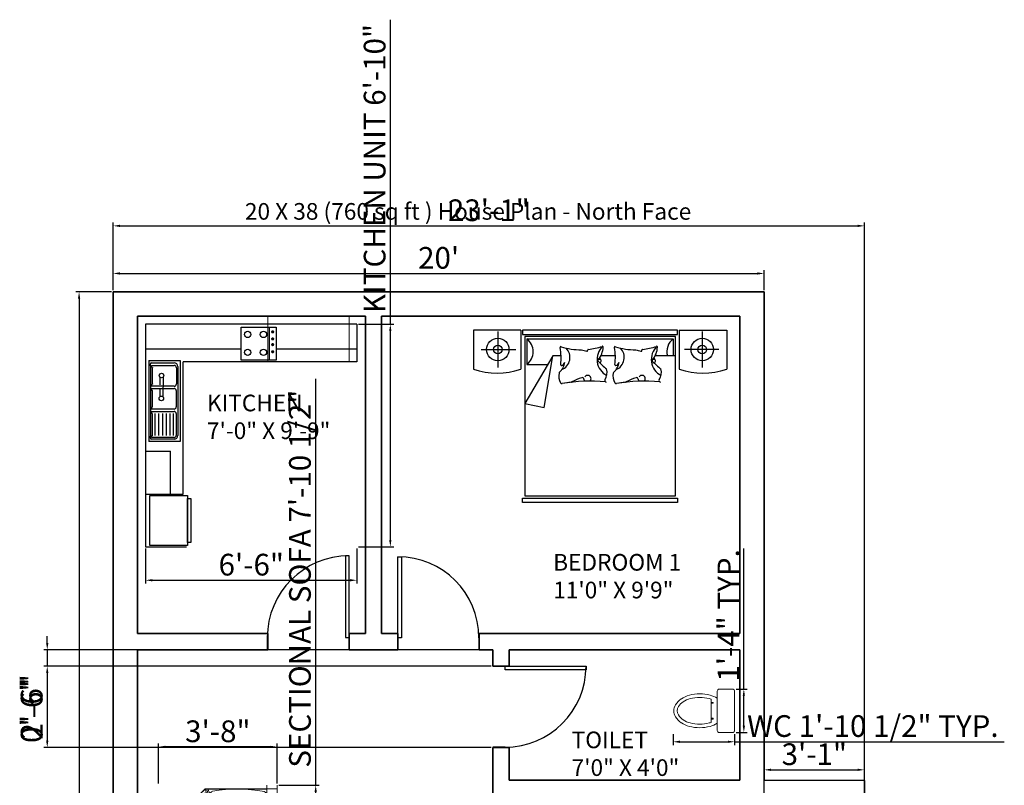
# Model space of a CAD drawing. Units: inches. Extents: x 3064 to 3427, y 2432 to 3115.
# Tile 3 of 3: x 3064 to 3427, y 2833 to 3115. Entities that reach past the tile are written whole.
import ezdxf

# ---------------------------------------------------------------- set-up
doc = ezdxf.new("R2010")
doc.units = ezdxf.units.IN
for name, color, linetype, lineweight in [('A-ANNO-DIMS', 2, 'Continuous', 13), ('A-ANNO-TEXT', 7, 'Continuous', 25), ('A-AREA-IDEN', 7, 'Continuous', 18), ('A-DOOR', 4, 'Continuous', 25), ('A-WALL', 7, 'Continuous', 35), ('FUR', 42, 'Continuous', 18), ('THIET-BI', 21, 'Continuous', 18)]:
    doc.layers.add(name, color=color, linetype=linetype, lineweight=lineweight)
for name, color, linetype in [('HID', 11, 'Continuous'), ('SAN', 5, 'Continuous'), ('TEFRIŞ', 11, 'Continuous'), ('wood', 26, 'Continuous')]:
    doc.layers.add(name, color=color, linetype=linetype)
doc.styles.get("Standard").update_dxf_attribs({"font": 'arial.ttf'})
doc.dimstyles.new('ISO-25', dxfattribs={"dimtxt": 8, "dimasz": 2.5, "dimexe": 1.25, "dimexo": 0.625, "dimtad": 1, "dimdec": 0, "dimlunit": 4, "dimtxsty": 'Standard', "dimcen": 2.5, "dimadec": 0, "dimazin": 0, "dimtfac": 1, "dimtdec": 0, "dimtmove": 0, "dimatfit": 3, "dimfxl": 1, "dimarcsym": 0})

# ---------------------------------------------------------------- blocks, each defined once
blk = doc.blocks.new('A$C008029BD')
at = {"layer": 'TEFRIŞ', "ltscale": 0.05}
for p, q in [((0, 0), (0, -3.55)), ((3.37, 0), (0, 0)), ((3.37, 0), (3.37, -0.6)), ((1.522, -0.4), (0, -0.4)), ((3.37, -0.4), (2.083, -0.4)), ((0.05, -0.581), (0.05, -1.869)), ((0.05, -0.581), (0.55, -0.581)), ((0.096, -0.617), (0.454, -0.617)), ((0.55, -0.581), (0.55, -1.869)), ((0.6, -2.71), (0.6, -0.6)), ((3.37, -0.6), (0.6, -0.6)), ((0.086, -1.773), (0.086, -0.677)), ((0.099, -0.659), (0.457, -0.659)), ((0.113, -0.954), (0.113, -0.695)), ((0.493, -0.695), (0.493, -0.954)), ((0.514, -0.677), (0.514, -1.773)), ((0.23, -0.846), (0.229, -0.967)), ((0.28, -0.846), (0.277, -1.158)), ((0.096, -1.024), (0.454, -1.024)), ((0.457, -0.99), (0.099, -0.99)), ((0.11, -1.319), (0.11, -1.06)), ((0.228, -1.02), (0.227, -1.159)), ((0.49, -1.06), (0.49, -1.319)), ((0.454, -1.355), (0.096, -1.355)), ((0.096, -1.391), (0.454, -1.391)), ((0.11, -1.773), (0.11, -1.427)), ((0.154, -1.773), (0.154, -1.427)), ((0.214, -1.773), (0.214, -1.427)), ((0.274, -1.773), (0.274, -1.427)), ((0.334, -1.773), (0.334, -1.427)), ((0.39, -1.773), (0.39, -1.427)), ((0.444, -1.773), (0.444, -1.427)), ((0.49, -1.427), (0.49, -1.773)), ((0.55, -1.869), (0.05, -1.869)), ((0.454, -1.809), (0.096, -1.809)), ((0.454, -1.833), (0.096, -1.833)), ((0, -2.025), (0.4, -2.025)), ((0.4, -2.71), (0.4, -2.025)), ((0, -2.71), (0.6, -2.71)), ((0, -3.55), (0.65, -3.55))]:
    blk.add_line(p, q, dxfattribs=at)
at = {"layer": 'TEFRIŞ'}
blk.add_line((1.969, -0.05), (1.969, -0.572), dxfattribs=at)
at = {"layer": 'TEFRIŞ', "ltscale": 0.05}
for points in [[(1.522, -0.05), (2.083, -0.05), (2.083, -0.572), (1.522, -0.572)], [(0.67, -2.73), (0.67, -3.53), (0.07, -3.53), (0.07, -2.73)], [(0.72, -2.78), (0.72, -3.48), (0.67, -3.48), (0.67, -2.78)]]:
    blk.add_lwpolyline(points, close=True, dxfattribs=at)
at = {"layer": 'TEFRIŞ', "const_width": 0.025}
for points in [[(2.014, -0.123, 1), (2.039, -0.123, 1)], [(2.014, -0.236, 1), (2.039, -0.236, 1)], [(2.014, -0.327, 1), (2.039, -0.327, 1)], [(2.014, -0.44, 1), (2.039, -0.44, 1)]]:
    blk.add_lwpolyline(points, format="xyb", close=True, dxfattribs=at)
at = {"layer": 'TEFRIŞ', "ltscale": 0.05}
for centre, radius in [((1.628, -0.164), 0.0505), ((1.628, -0.45), 0.0505), ((0.255, -0.82), 0.036), ((0.252, -1.184), 0.036)]:
    blk.add_circle(centre, radius, dxfattribs=at)
at = {"layer": 'TEFRIŞ'}
for centre in [(1.88, -0.164), (1.88, -0.45)]:
    blk.add_circle(centre, 0.0505, dxfattribs=at)
at = {"layer": 'TEFRIŞ', "ltscale": 0.05}
for centre, radius, start, end in [((0.108, -0.649), 0.0351, 110.4976, 230.5777), ((0.454, -0.677), 0.06, 0, 90), ((0.118, -0.673), 0.023, 143.9853, 258.5157), ((0.457, -0.695), 0.036, 0, 90), ((0.115, -1.038), 0.023, 143.9853, 258.5157), ((0.118, -0.976), 0.023, 101.4843, 216.0147), ((0.454, -1.06), 0.036, 0, 90), ((0.457, -0.954), 0.036, 270, 0), ((0.115, -1.341), 0.023, 101.4843, 216.0147), ((0.115, -1.405), 0.023, 143.9853, 258.5157), ((0.454, -1.319), 0.036, 270, 0), ((0.454, -1.427), 0.036, 0, 90), ((0.108, -1.801), 0.0351, 129.4223, 249.5024), ((0.115, -1.796), 0.023, 101.4843, 216.0147), ((0.454, -1.773), 0.06, 270, 0), ((0.454, -1.773), 0.036, 270, 0)]:
    blk.add_arc(centre, radius, start, end, dxfattribs=at)
blk = doc.blocks.new('A$C47AC156F')
at = {"layer": 'HID'}
for centre, radius, start, end in [((1.015, 1.799), 0.00933, 72.7248, 190.959), ((0.396, 1.679), 0.622, 352.7363, 10.959), ((1.25, 2.553), 0.781, 252.7248, 270.2702), ((0.966, 1.684), 0.155, 292.7628, 43.8922), ((1.385, 2.121), 0.373, 249.4168, 259.3085), ((1.317, 1.764), 0.00933, 259.3085, 10.689), ((1.336, 1.768), 0.00933, 96.2196, 190.689), ((1.25, 2.553), 0.781, 276.2196, 288.2114), ((1.645, 1.66), 0.21, 133.8947, 242.3952), ((1.258, 1.815), 0.249, 319.9211, 357.124), ((1.497, 1.803), 0.00933, 357.124, 108.2114), ((1.497, 1.803), 0.00933, 357.124, 108.2114), ((1.645, 1.799), 0.00933, 72.7248, 190.959), ((1.026, 1.679), 0.622, 352.7363, 10.959), ((1.88, 2.553), 0.781, 252.7248, 270.2702), ((1.596, 1.684), 0.155, 292.7628, 43.8922), ((2.015, 2.121), 0.373, 249.4168, 259.3085), ((1.947, 1.764), 0.00933, 259.3085, 10.689), ((1.966, 1.768), 0.00933, 96.2196, 190.689), ((1.88, 2.553), 0.781, 276.2196, 288.2114), ((2.275, 1.66), 0.21, 133.8947, 242.3952), ((1.888, 1.815), 0.249, 319.9211, 357.124), ((2.127, 1.803), 0.00933, 357.124, 108.2114), ((2.127, 1.803), 0.00933, 357.124, 108.2114), ((0.871, 1.658), 0.194, 311.6071, 349.7845), ((1.005, 1.648), 0.0615, 288.2985, 335.7891), ((1.453, 1.646), 0.00933, 118.8315, 225.8329), ((2.727, 2.958), 1.838, 225.8329, 230.0245), ((0.994, -0.376), 2.088, 76.4982, 77.2888), ((0.994, 3.644), 2.088, 282.7018, 282.7206), ((1.445, 1.644), 0.0373, 312.662, 59.1573), ((1.501, 1.658), 0.194, 311.6071, 349.7845), ((1.635, 1.648), 0.0615, 288.2985, 335.7891), ((2.083, 1.646), 0.00933, 118.8315, 225.8329), ((3.357, 2.958), 1.838, 225.8329, 230.0245), ((1.624, -0.376), 2.088, 76.4982, 77.2888), ((1.624, 3.644), 2.088, 282.7018, 282.7206), ((2.075, 1.644), 0.0373, 312.662, 59.1573), ((1.142, 1.469), 0.152, 167.3377, 211.666), ((1.012, 1.499), 0.0187, 131.6071, 167.3377), ((1.022, 1.599), 0.00933, 172.7363, 288.2985), ((1.401, 1.508), 0.151, 327.1663, 15.7613), ((1.772, 1.469), 0.152, 167.3377, 211.666), ((1.642, 1.499), 0.0187, 131.6071, 167.3377), ((1.652, 1.599), 0.00933, 172.7363, 288.2985), ((2.031, 1.508), 0.151, 327.1663, 15.7613), ((1.028, 1.399), 0.0187, 211.666, 279.4465), ((1.35, -0.534), 1.941, 84.5852, 99.4465), ((1.35, -0.534), 1.941, 96.386, 99.4465), ((1.132, 1.414), 0.0187, 276.386, 303.7955), ((1.54, 0.631), 0.864, 109.049, 117.3823), ((1.264, 1.43), 0.0187, 2.6426, 109.049), ((1.301, 1.432), 0.0187, 182.6426, 192.7015), ((1.323, 1.437), 0.0414, 192.7015, 227.1556), ((1.326, 1.436), 0.0395, 312.3565, 145.7762), ((1.543, 1.416), 0.0187, 147.1663, 264.3422), ((1.659, 1.399), 0.0187, 211.666, 279.4465), ((1.98, -0.534), 1.941, 84.5852, 99.4465), ((1.98, -0.534), 1.941, 96.386, 99.4465), ((1.762, 1.414), 0.0187, 276.386, 303.7955), ((2.17, 0.631), 0.864, 109.049, 117.3823), ((1.894, 1.43), 0.0187, 2.6426, 109.049), ((1.931, 1.432), 0.0187, 182.6426, 192.7015), ((1.954, 1.437), 0.0414, 192.7015, 227.1556), ((1.956, 1.436), 0.0395, 312.3565, 145.7762), ((2.173, 1.416), 0.0187, 147.1663, 264.3422)]:
    blk.add_arc(centre, radius, start, end, dxfattribs=at)
at = {"layer": 'SAN'}
for p, q in [((0.283, 1.985), (0.283, 1.566)), ((2.657, 1.985), (2.657, 1.566)), ((0.09, 1.775), (0.491, 1.775)), ((2.85, 1.775), (2.449, 1.775))]:
    blk.add_line(p, q, dxfattribs=at)
for centre, radius in [((0.283, 1.775), 0.13), ((2.657, 1.775), 0.13), ((0.283, 1.775), 0.05), ((2.657, 1.775), 0.05)]:
    blk.add_circle(centre, radius, dxfattribs=at)
at = {"layer": 'wood'}
for p, q in [((0, 1.998), (0, 1.548)), ((0.55, 1.998), (0, 1.998)), ((0.55, 1.998), (0.55, 1.548)), ((2.39, 1.998), (2.94, 1.998)), ((2.39, 1.998), (2.39, 1.548)), ((2.94, 1.998), (2.94, 1.548)), ((0.62, 1.9), (2.32, 1.9)), ((0.62, 1.9), (0.62, 1.6)), ((2.32, 1.9), (2.32, 1.7)), ((0.92, 1.7), (0.595, 1.15)), ((0.82, 1.1), (0.92, 1.7)), ((1.017, 1.7), (0.92, 1.7)), ((1.647, 1.7), (1.479, 1.7)), ((2.345, 1.7), (2.109, 1.7)), ((0.62, 1.6), (0.861, 1.6)), ((0.595, 1.15), (0.82, 1.1))]:
    blk.add_line(p, q, dxfattribs=at)
for points in [[(0.57, 1.95), (2.37, 1.95), (2.37, 2), (0.57, 2)], [(2.345, 0.075), (2.345, 1.925), (0.595, 1.925), (0.595, 0.075)], [(0.57, 0.05), (2.37, 0.05), (2.37, 0), (0.57, 0)]]:
    blk.add_lwpolyline(points, close=True, dxfattribs=at)
for centre, radius, start, end in [((0.504, 1.75), 0.19, 307.7826, 52.2174), ((2.436, 1.75), 0.19, 127.7826, 195.2747), ((0.275, 2.342), 0.84, 250.89, 289.11), ((2.665, 2.342), 0.84, 250.89, 289.11)]:
    blk.add_arc(centre, radius, start, end, dxfattribs=at)
blk = doc.blocks.new('A$C5B9B1B1E')
at = {"layer": 'FUR'}
for p, q in [((0.68, 1.857), (3.32, 1.857)), ((0.044, 1.127), (0.687, 1.804)), ((0.046, 1.126), (0.691, 1.805)), ((0.687, 1.804), (3.246, 1.804)), ((0.689, 1.807), (3.298, 1.807)), ((0.718, 1.807), (1.035, 0.991)), ((0.741, 1.807), (0.774, 1.719)), ((1.587, 1.804), (1.587, 1.757)), ((1.608, 1.804), (1.608, 1.041)), ((1.629, 1.804), (1.629, 1.757)), ((2.343, 1.804), (2.343, 1.041)), ((2.364, 1.804), (2.364, 1.041)), ((2.385, 1.804), (2.385, 1.757)), ((3.27, 1.807), (2.952, 0.991)), ((3.247, 1.807), (3.213, 1.719)), ((3.942, 1.126), (3.296, 1.805)), ((3.944, 1.127), (3.298, 1.807)), ((0.748, 1.672), (1.007, 1.005)), ((0.792, 1.675), (1.057, 0.993)), ((1.587, 1.671), (1.587, 1.041)), ((1.603, 1.671), (1.603, 1.041)), ((1.629, 1.671), (1.629, 1.041)), ((2.385, 1.671), (2.385, 1.041)), ((3.196, 1.675), (2.93, 0.993)), ((3.24, 1.672), (2.98, 1.005)), ((0.044, 1.127), (0.044, 0)), ((0.044, 1.127), (0.112, 1.103)), ((0.044, 1.105), (0.856, 0.808)), ((0.044, 1.083), (0.133, 1.05)), ((0.046, 1.082), (0.046, 0.164)), ((0.181, 1.077), (0.842, 0.836)), ((3.944, 1.105), (3.131, 0.808)), ((3.807, 1.077), (3.145, 0.836)), ((3.944, 1.083), (3.854, 1.05)), ((3.944, 1.127), (3.875, 1.103)), ((3.941, 1.082), (3.941, 0.164)), ((3.944, 1.127), (3.944, 0)), ((0.167, 1.038), (0.86, 0.785)), ((0.997, 0.952), (0.895, 0.848)), ((2.991, 0.952), (3.093, 0.848)), ((3.82, 1.038), (3.128, 0.785)), ((0, 0.164), (0.663, 0.164)), ((4, 0.164), (3.325, 0.164)), ((0, 0), (0.775, 0)), ((4, 0), (3.219, 0))]:
    blk.add_line(p, q, dxfattribs=at)
for centre, radius, start, end in [((1.999, -0.1), 2.263, 125.9311, 146.4201), ((0.827, 1.714), 0.0525, 104.0803, 255.9197), ((1.2, -0.267), 2.068, 79.3218, 100.7558), ((1.571, 1.714), 0.0529, 283.4421, 76.5579), ((1.661, 1.714), 0.0529, 103.4421, 256.5579), ((1.974, 0.302), 1.499, 77.3591, 102.5496), ((2.289, 1.714), 0.0525, 284.0803, 75.9197), ((2.417, 1.714), 0.0529, 103.4421, 256.5579), ((2.788, -0.267), 2.068, 79.2442, 100.6782), ((3.161, 1.714), 0.0525, 284.0803, 75.9197), ((1.989, -0.1), 2.263, 33.5799, 54.0689), ((-2.245, 3.806), 3.68, 319.5649, 324.3474), ((-2.245, 3.806), 3.733, 320.6889, 324.3474), ((1.373, 5.964), 4.337, 262.5873, 266.2564), ((1.493, 7.461), 5.886, 263.3874, 265.2569), ((1.257, 3.126), 1.499, 272.4014, 282.5496), ((1.257, 3.126), 1.551, 272.4014, 282.5496), ((1.974, 3.126), 1.551, 257.1404, 261.9048), ((1.974, 3.126), 1.499, 257.4504, 262.6454), ((1.974, 3.126), 1.499, 274.5548, 275.3997), ((1.974, 3.126), 1.499, 278.9885, 282.6409), ((1.974, 3.126), 1.551, 280.7847, 283.7486), ((2.73, 3.126), 1.551, 257.4504, 267.5986), ((2.73, 3.126), 1.499, 257.4504, 267.5986), ((2.614, 5.964), 4.337, 273.7436, 277.4127), ((2.494, 7.461), 5.886, 274.7431, 276.6126), ((6.233, 3.806), 3.733, 215.6526, 219.3111), ((6.233, 3.806), 3.68, 215.6526, 220.4351), ((0.159, 1.125), 0.0525, 149.9951, 301.8345), ((-0.635, 2.334), 1.499, 303.2739, 311.5982), ((-0.635, 2.334), 1.551, 304.4606, 312.1941), ((4.623, 2.334), 1.551, 227.8059, 235.5394), ((4.623, 2.334), 1.499, 228.4018, 236.7261), ((3.828, 1.125), 0.0525, 238.1655, 30.0049), ((2.31, 0.617), 2.263, 170.0163, 190.5053), ((0.133, 0.997), 0.0529, 13.4421, 166.5579), ((-3.456, 0.47), 3.68, 1.9572, 8.4326), ((-3.456, 0.47), 3.733, 1.9572, 8.4326), ((0.961, 0.987), 0.05, 315.6002, 21.264), ((1.299, 2.034), 1.068, 256.9274, 284.5801), ((1.545, 1.041), 0.042, 279.7794, 0), ((1.561, 1.041), 0.042, 279.7794, 0), ((1.671, 1.041), 0.042, 180, 260.2206), ((1.986, 2.869), 1.897, 260.2206, 279.7794), ((2.301, 1.041), 0.042, 279.7794, 0), ((2.427, 1.041), 0.042, 180, 260.2206), ((2.689, 2.034), 1.068, 255.4199, 283.0726), ((3.027, 0.987), 0.05, 158.736, 224.3998), ((7.443, 0.47), 3.733, 171.5674, 178.0428), ((7.443, 0.47), 3.68, 171.5674, 178.0428), ((3.854, 0.997), 0.0529, 13.4421, 166.5579), ((1.678, 0.617), 2.263, 349.4947, 9.9837), ((-1.061, 0.519), 1.939, 345.4239, 7.8665), ((0.859, 0.883), 0.05, 249.9365, 315.6002), ((3.128, 0.883), 0.05, 224.3998, 290.0635), ((5.006, 0.521), 1.897, 172.0077, 194.7607), ((-1.275, 0.533), 1.499, 347.3591, 353.601), ((5.263, 0.533), 1.499, 186.399, 192.6409), ((0.136, 0.218), 0.0525, 194.0803, 345.9197), ((-1.275, 0.533), 1.551, 346.2514, 350.7022), ((0.643, 0.074), 0.0918, 328.6411, 77.5888), ((3.345, 0.074), 0.0918, 102.4112, 211.3589), ((5.263, 0.533), 1.551, 189.2978, 193.7486), ((3.851, 0.218), 0.0525, 194.0803, 345.9197), ((0.665, 0.069), 0.0703, 279.5212, 322.6757), ((0.775, 0.042), 0.042, 270, 345.2393), ((3.226, 0.057), 0.0573, 199.356, 262.7582), ((3.338, 0.086), 0.0936, 219.4969, 247.1448)]:
    blk.add_arc(centre, radius, start, end, dxfattribs=at)
at = {"layer": 'HID'}
for centre, radius, start, end in [((1.056, 2.162), 0.527, 287.478, 299.4698), ((1.393, 1.632), 0.104, 135.6927, 273.5175), ((1.159, 1.674), 0.168, 330.4242, 8.3824), ((1.319, 1.698), 0.0063, 8.3824, 119.4698), ((1.664, 1.652), 0.142, 287.6048, 36.1053), ((1.94, 1.709), 0.168, 172.876, 210.0789), ((1.78, 1.729), 0.0063, 61.7886, 172.876), ((1.78, 1.729), 0.0063, 61.7886, 172.876), ((2.032, 2.199), 0.527, 241.7886, 253.7804), ((1.883, 1.687), 0.0063, 339.311, 73.7804), ((2.283, 1.626), 0.168, 151.6176, 189.5758), ((2.141, 1.703), 0.0063, 40.5302, 151.6176), ((2.546, 2.05), 0.527, 220.5302, 232.522), ((2.594, 1.632), 0.104, 266.4825, 44.3073), ((2.829, 1.674), 0.168, 171.6176, 209.5758), ((2.669, 1.698), 0.0063, 60.5302, 171.6176), ((2.931, 2.162), 0.527, 240.5302, 252.522), ((1, 1.632), 0.0063, 83.9832, 202.2174), ((0.606, 1.471), 0.42, 3.9947, 22.2174), ((1.056, 2.162), 0.527, 263.9832, 281.5286), ((0.982, 1.549), 0.105, 304.0212, 55.1506), ((1.202, 1.894), 0.252, 260.6752, 270.5669), ((1.205, 1.649), 0.0063, 270.5669, 21.9475), ((1.216, 1.653), 0.0063, 107.478, 201.9475), ((1.31, 1.588), 0.0063, 150.4242, 237.1103), ((1.981, 2.625), 1.241, 237.1103, 241.1368), ((1.379, 1.514), 0.0244, 343.8009, 85.0524), ((1.809, 1.522), 0.102, 154.2387, 202.8337), ((1.795, 1.618), 0.0252, 110.8427, 217.338), ((1.859, 0.222), 1.409, 92.7112, 93.5018), ((2.33, 2.894), 1.409, 247.2794, 247.2982), ((1.791, 1.62), 0.0063, 304.1671, 51.1685), ((1.895, 1.683), 0.0063, 159.311, 270.6915), ((1.892, 1.928), 0.252, 270.6915, 280.5832), ((2.032, 2.199), 0.527, 259.7298, 277.2752), ((2.009, 1.552), 0.0126, 176.1991, 230.6607), ((2.302, 1.91), 0.476, 230.6607, 243.8744), ((2.119, 1.588), 0.105, 126.1078, 237.2372), ((2.088, 1.569), 0.0416, 194.2109, 241.7015), ((2.179, 1.559), 0.131, 180.2155, 218.3929), ((2.072, 1.538), 0.0063, 241.7015, 357.2637), ((2.497, 1.518), 0.42, 159.041, 177.2637), ((2.099, 1.67), 0.0063, 339.041, 97.2752), ((2.111, 1.597), 0.0063, 282.8897, 9.5758), ((2.231, 1.618), 0.0063, 138.0525, 249.4331), ((2.222, 1.627), 0.0063, 318.0525, 52.522), ((2.317, 1.848), 0.252, 249.4331, 259.3248), ((2.546, 2.05), 0.527, 238.4714, 256.0168), ((2.406, 1.449), 0.105, 104.8494, 215.9788), ((2.417, 1.532), 0.0063, 317.7826, 76.0168), ((2.608, 1.514), 0.0244, 94.9476, 196.1991), ((2.007, 2.625), 1.241, 298.8632, 302.8897), ((2.677, 1.588), 0.0063, 302.8897, 29.5758), ((2.771, 1.653), 0.0063, 338.0525, 72.522), ((2.783, 1.649), 0.0063, 158.0525, 269.4331), ((2.785, 1.894), 0.252, 269.4331, 279.3248), ((2.931, 2.162), 0.527, 258.4714, 276.0168), ((3.005, 1.549), 0.105, 124.8494, 235.9788), ((3.382, 1.471), 0.42, 157.7826, 176.0053), ((2.987, 1.632), 0.0063, 337.7826, 96.0168), ((0.277, 1.564), 0.252, 306.59, 316.4817), ((0.459, 1.407), 0.0063, 153.3928, 247.8623), ((-0.018, 1.646), 0.527, 333.3928, 345.3846), ((0.455, 1.395), 0.0063, 316.4817, 67.8623), ((0.498, 1.511), 0.0063, 54.2972, 165.3846), ((0.598, 1.519), 0.104, 181.6075, 319.4323), ((0.404, 1.38), 0.168, 16.339, 54.2972), ((0.571, 1.429), 0.0063, 196.339, 283.0251), ((0.293, 2.632), 1.241, 283.0251, 287.0516), ((0.263, 1.627), 0.476, 322.0404, 335.2541), ((0.673, 1.427), 0.0244, 29.7157, 130.9672), ((0.683, 1.433), 0.0126, 335.2541, 29.7157), ((1.031, 1.5), 0.0063, 183.9947, 299.557), ((1.013, 1.531), 0.0416, 299.557, 347.0475), ((0.923, 1.519), 0.131, 329.5087, 1.0429), ((1.135, 1.458), 0.099, 182.7962, 207.1304), ((1.058, 1.418), 0.0126, 207.1304, 290.9482), ((1.531, 0.183), 1.31, 105.1521, 110.9482), ((1.185, 1.46), 0.0126, 285.1521, 322.4345), ((1.324, 1.352), 0.163, 100.921, 142.4345), ((1.274, 1.728), 0.252, 258.5381, 270.9308), ((1.286, 1.487), 0.0126, 131.4659, 280.4525), ((1.185, 1.602), 0.141, 311.4659, 320.8131), ((1.237, 1.948), 0.476, 276.1256, 289.3393), ((1.391, 1.511), 0.0126, 289.3393, 343.8009), ((1.704, 1.478), 0.0126, 265.6578, 22.8337), ((1.603, 0.159), 1.31, 70.5535, 85.4148), ((1.85, 1.466), 0.0267, 24.2238, 217.6435), ((1.852, 1.466), 0.0279, 302.8444, 337.2985), ((1.866, 1.46), 0.0126, 337.2985, 347.3574), ((1.891, 1.454), 0.0126, 60.951, 167.3574), ((1.614, 0.955), 0.583, 52.6177, 60.951), ((1.977, 1.428), 0.0126, 226.2045, 253.614), ((1.603, 0.159), 1.31, 70.5535, 73.614), ((2.044, 1.406), 0.0126, 250.5535, 318.334), ((1.976, 1.466), 0.103, 318.334, 2.6623), ((2.067, 1.47), 0.0126, 2.6623, 38.3929), ((2.099, 1.494), 0.0126, 239.5475, 28.5341), ((2.234, 1.567), 0.141, 199.1869, 208.5341), ((2.017, 1.381), 0.163, 17.5655, 59.079), ((2.193, 1.717), 0.252, 249.0692, 261.4619), ((2.185, 1.434), 0.0126, 197.5655, 234.8479), ((1.423, 0.352), 1.31, 49.0518, 54.8479), ((2.452, 1.4), 0.131, 158.9571, 190.4913), ((2.371, 1.442), 0.0416, 172.9525, 220.443), ((2.344, 1.419), 0.0063, 220.443, 336.0053), ((2.733, 1.246), 0.42, 137.7826, 156.0053), ((2.597, 1.511), 0.0126, 196.1991, 250.6607), ((2.75, 1.948), 0.476, 250.6607, 263.8744), ((2.663, 1.352), 0.163, 37.5655, 79.079), ((2.803, 1.602), 0.141, 219.1869, 228.5341), ((2.702, 1.487), 0.0126, 259.5475, 48.5341), ((2.713, 1.728), 0.252, 269.0692, 281.4619), ((2.803, 1.46), 0.0126, 217.5655, 254.8479), ((2.457, 0.183), 1.31, 69.0518, 74.8479), ((2.93, 1.418), 0.0126, 249.0518, 332.8696), ((3.065, 1.519), 0.131, 178.9571, 210.4913), ((2.974, 1.531), 0.0416, 192.9525, 240.443), ((2.853, 1.458), 0.099, 332.8696, 357.2038), ((2.957, 1.5), 0.0063, 240.443, 356.0053), ((3.304, 1.433), 0.0126, 150.2843, 204.7459), ((3.315, 1.427), 0.0244, 49.0328, 150.2843), ((3.725, 1.627), 0.476, 204.7459, 217.9596), ((3.389, 1.519), 0.104, 220.5677, 358.3925), ((3.694, 2.632), 1.241, 252.9484, 256.9749), ((3.416, 1.429), 0.0063, 256.9749, 343.661), ((3.583, 1.38), 0.168, 125.7028, 163.661), ((4.005, 1.646), 0.527, 194.6154, 206.6072), ((3.533, 1.395), 0.0063, 112.1377, 223.5183), ((3.711, 1.564), 0.252, 223.5183, 233.41), ((3.528, 1.407), 0.0063, 292.1377, 26.6072), ((0.371, 1.166), 0.105, 349.936, 101.0654), ((1.734, 0.609), 1.31, 151.0669, 156.863), ((0.751, 1.275), 0.163, 146.8358, 188.3493), ((0.446, 1.501), 0.252, 304.4529, 316.8456), ((0.577, 1.249), 0.0126, 331.0669, 8.3493), ((0.474, 1.348), 0.141, 357.3807, 6.7279), ((0.627, 1.341), 0.0126, 177.3807, 326.3673), ((2.29, 1.351), 0.0126, 229.0518, 312.8696), ((2.232, 1.415), 0.099, 312.8696, 337.2038), ((3.36, 1.341), 0.0126, 213.6327, 2.6193), ((3.542, 1.501), 0.252, 223.1544, 235.5471), ((3.513, 1.348), 0.141, 173.2721, 182.6193), ((3.237, 1.275), 0.163, 351.6507, 33.1642), ((3.411, 1.249), 0.0126, 171.6507, 208.9331), ((2.253, 0.609), 1.31, 23.137, 28.9331), ((3.616, 1.166), 0.105, 78.9346, 190.064), ((3.822, 0.841), 0.42, 111.8678, 130.0905), ((4.005, 1.646), 0.527, 212.5566, 230.102), ((0.44, 1.167), 0.0063, 229.9095, 345.4718), ((0.406, 1.176), 0.0416, 345.4718, 32.9623), ((0.351, 1.103), 0.131, 15.4235, 46.9577), ((0.543, 1.212), 0.099, 228.711, 253.0452), ((0.518, 1.129), 0.0126, 253.0452, 336.863), ((3.47, 1.129), 0.0126, 203.137, 286.9548), ((3.445, 1.212), 0.099, 286.9548, 311.289), ((3.636, 1.103), 0.131, 133.0423, 164.5765), ((3.582, 1.176), 0.0416, 147.0377, 194.5282), ((3.547, 1.167), 0.0063, 194.5282, 310.0905), ((0.219, 0.669), 0.104, 225.6927, 3.5175), ((-0.775, 1.256), 1.241, 327.1103, 331.1368), ((0.336, 0.655), 0.0244, 73.8009, 175.0524), ((0.34, 0.666), 0.0126, 19.3393, 73.8009), ((-0.097, 0.513), 0.476, 6.1256, 19.3393), ((4.085, 0.513), 0.476, 160.6607, 173.8744), ((3.648, 0.666), 0.0126, 106.1991, 160.6607), ((3.651, 0.655), 0.0244, 4.9476, 106.1991), ((3.769, 0.669), 0.104, 176.4825, 314.3073), ((4.762, 1.256), 1.241, 208.8632, 212.8897), ((0.152, 0.594), 0.0063, 98.3824, 209.4698), ((-0.312, 0.331), 0.527, 17.478, 29.4698), ((0.176, 0.434), 0.168, 60.4242, 98.3824), ((0.197, 0.492), 0.0063, 197.478, 291.9475), ((0.202, 0.48), 0.0063, 0.5669, 111.9475), ((-0.044, 0.478), 0.252, 350.6752, 0.5669), ((0.262, 0.586), 0.0063, 240.4242, 327.1103), ((0.498, 0.6), 0.163, 190.921, 232.4345), ((0.249, 0.46), 0.141, 41.4659, 50.8131), ((0.363, 0.561), 0.0126, 221.4659, 10.4525), ((0.122, 0.55), 0.252, 348.5381, 0.9308), ((0.391, 0.46), 0.0126, 15.1521, 52.4345), ((1.668, 0.806), 1.31, 195.1521, 200.9482), ((2.32, 0.806), 1.31, 339.0518, 344.8479), ((3.597, 0.46), 0.0126, 127.5655, 164.8479), ((3.49, 0.6), 0.163, 307.5655, 349.079), ((3.624, 0.561), 0.0126, 169.5475, 318.5341), ((3.866, 0.55), 0.252, 179.0692, 191.4619), ((3.739, 0.46), 0.141, 129.1869, 138.5341), ((3.726, 0.586), 0.0063, 212.8897, 299.5758), ((3.811, 0.434), 0.168, 81.6176, 119.5758), ((3.786, 0.48), 0.0063, 68.0525, 179.4331), ((4.031, 0.478), 0.252, 179.4331, 189.3248), ((3.791, 0.492), 0.0063, 248.0525, 342.522), ((4.3, 0.331), 0.527, 150.5302, 162.522), ((-0.312, 0.331), 0.527, 353.9832, 11.5286), ((0.301, 0.258), 0.105, 34.0212, 145.1506), ((0.319, 0.289), 0.0416, 29.557, 77.0475), ((0.331, 0.198), 0.131, 59.5087, 91.0429), ((0.35, 0.306), 0.0063, 273.9947, 29.557), ((0.393, 0.41), 0.099, 272.7962, 297.1304), ((0.432, 0.333), 0.0126, 297.1304, 20.9482), ((3.556, 0.333), 0.0126, 159.0518, 242.8696), ((3.595, 0.41), 0.099, 242.8696, 267.2038), ((3.657, 0.198), 0.131, 88.9571, 120.4913), ((3.687, 0.258), 0.105, 34.8494, 145.9788), ((3.638, 0.306), 0.0063, 150.443, 266.0053), ((3.668, 0.289), 0.0416, 102.9525, 150.443), ((4.3, 0.331), 0.527, 168.4714, 186.0168), ((0.219, 0.276), 0.0063, 173.9832, 292.2174), ((0.38, -0.119), 0.42, 93.9947, 112.2174), ((3.608, -0.119), 0.42, 67.7826, 86.0053), ((3.769, 0.276), 0.0063, 247.7826, 6.0168)]:
    blk.add_arc(centre, radius, start, end, dxfattribs=at)
blk = doc.blocks.new('*D6')
at = {"layer": 'A-ANNO-DIMS', "color": 0, "lineweight": -2, "transparency": 16777216}
for p, q in [((3338.05, 2829.08), (3338.05, 2839.48)), ((3375.05, 2829.08), (3375.05, 2839.48)), ((3340.55, 2838.23), (3372.55, 2838.23))]:
    blk.add_line(p, q, dxfattribs=at)
at = {"layer": 'A-ANNO-DIMS', "color": 0, "transparency": 16777216}
for points in [[(3340.55, 2838.65), (3340.55, 2837.82), (3338.05, 2838.23)], [(3372.55, 2838.65), (3372.55, 2837.82), (3375.05, 2838.23)]]:
    blk.add_solid(points, dxfattribs=at)
at = {"layer": 'Defpoints', "color": 0, "transparency": 16777216}
for p in [(3375.05, 2838.23), (3338.05, 2828.45), (3375.05, 2828.45)]:
    blk.add_point(p, dxfattribs=at)
at = {"layer": 'A-ANNO-DIMS', "color": 0, "transparency": 16777216, "insert": (3356.55, 2842.95), "char_height": 8, "attachment_point": 5}
blk.add_mtext('3\'-1"', dxfattribs=at)
blk = doc.blocks.new('*U10')
for p, q in [((0, 0), (0, -6)), ((40, 0), (40, -6))]:
    blk.add_line(p, q)
blk.add_lwpolyline([(0, 0), (0, 40), (1.75, 40), (1.75, 0)], close=True)
blk.add_arc((0, 0), 40, 0, 90)
blk = doc.blocks.new('*U11')
for p, q in [((0, 0), (0, -6)), ((-40, 0), (-40, -6))]:
    blk.add_line(p, q)
blk.add_lwpolyline([(0, 0), (0, 40), (-1.75, 40), (-1.75, 0)], close=True)
blk.add_arc((0, 0), 40, 90, 180)
blk = doc.blocks.new('*U14')
for p, q in [((-40, 0), (-40, 6)), ((0, 0), (0, 6))]:
    blk.add_line(p, q)
blk.add_lwpolyline([(0, 0), (0, -40), (-1.75, -40), (-1.75, 0)], close=True)
blk.add_arc((0, 0), 40, 180, 270)
blk = doc.blocks.new('*D15')
at = {"layer": 'A-ANNO-DIMS', "color": 0, "lineweight": -2, "transparency": 16777216}
for p, q in [((3098.05, 3015.08), (3098.05, 3022.44)), ((3100.55, 3021.19), (3335.55, 3021.19)), ((3338.05, 3015.08), (3338.05, 3022.44))]:
    blk.add_line(p, q, dxfattribs=at)
at = {"layer": 'A-ANNO-DIMS', "color": 0, "transparency": 16777216}
for points in [[(3100.55, 3021.61), (3100.55, 3020.77), (3098.05, 3021.19)], [(3335.55, 3021.61), (3335.55, 3020.77), (3338.05, 3021.19)]]:
    blk.add_solid(points, dxfattribs=at)
at = {"layer": 'Defpoints', "color": 0, "transparency": 16777216}
for p in [(3338.05, 3021.19), (3098.05, 3014.45), (3338.05, 3014.45)]:
    blk.add_point(p, dxfattribs=at)
at = {"layer": 'A-ANNO-DIMS', "color": 0, "transparency": 16777216, "insert": (3218.05, 3025.9), "char_height": 8, "attachment_point": 5}
blk.add_mtext("20'", dxfattribs=at)
blk = doc.blocks.new('*D16')
at = {"layer": 'A-ANNO-DIMS', "color": 0, "lineweight": -2, "transparency": 16777216}
for p, q in [((3097.42, 3014.45), (3084.25, 3014.45)), ((3085.5, 3011.95), (3085.5, 2560.95)), ((3097.42, 2558.45), (3084.25, 2558.45))]:
    blk.add_line(p, q, dxfattribs=at)
at = {"layer": 'A-ANNO-DIMS', "color": 0, "transparency": 16777216}
for points in [[(3085.09, 3011.95), (3085.92, 3011.95), (3085.5, 3014.45)], [(3085.09, 2560.95), (3085.92, 2560.95), (3085.5, 2558.45)]]:
    blk.add_solid(points, dxfattribs=at)
at = {"layer": 'Defpoints', "color": 0, "transparency": 16777216}
for p in [(3098.05, 3014.45), (3085.5, 2558.45), (3098.05, 2558.45)]:
    blk.add_point(p, dxfattribs=at)
at = {"layer": 'A-ANNO-DIMS', "color": 0, "transparency": 16777216, "insert": (3080.79, 2786.45), "char_height": 8, "attachment_point": 5, "rotation": 90}
blk.add_mtext("38'", dxfattribs=at)
blk = doc.blocks.new('WC-TANK')
for p, q in [((16.04, 15.24), (16.04, 0.8)), ((21.66, 16.04), (16.85, 16.04)), ((22.46, 0.8), (22.46, 15.24)), ((13.79, 11.11), (13.79, 10.8)), ((14.52, 11.11), (13.79, 11.11)), ((13.8, 12.29), (13.8, 3.76)), ((14.52, 10.8), (14.52, 11.11)), ((13.79, 10.8), (14.52, 10.8)), ((13.79, 4.94), (13.79, 5.26)), ((13.79, 5.26), (14.52, 5.26)), ((14.52, 4.94), (13.79, 4.94)), ((14.52, 5.26), (14.52, 4.94)), ((16.85, 0), (21.66, 0))]:
    blk.add_line(p, q)
for centre, radius, start, end in [((16.85, 15.24), 0.802, 90, 180), ((21.66, 15.24), 0.802, 0, 90), ((6.75, 6.36), 7.24, 123.0315, 147.5002), ((6.75, 6.36), 5.95, 123.0315, 147.5002), ((8.47, 3.73), 10.38, 105.0731, 123.0315), ((8.47, 3.73), 9.1, 105.0731, 123.0315), ((9.59, -0.44), 14.7, 74.9269, 105.0732), ((9.59, -0.44), 13.41, 74.9269, 105.0732), ((10.71, 3.73), 9.1, 70.176, 74.9269), ((10.71, 3.73), 10.38, 59.0966, 74.9269), ((4.15, 8.02), 4.15, 147.5002, 212.4998), ((4.15, 8.02), 2.87, 147.5002, 212.4998), ((6.75, 9.68), 7.24, 212.4998, 236.9685), ((6.75, 9.68), 5.95, 212.4998, 236.9685), ((8.47, 12.31), 9.1, 236.9685, 254.9269), ((10.71, 12.31), 9.1, 285.0731, 289.824), ((8.47, 12.31), 10.38, 236.9685, 254.9269), ((9.59, 16.48), 14.7, 254.9269, 285.0731), ((9.59, 16.48), 13.41, 254.9269, 285.0731), ((10.71, 12.31), 10.38, 285.0731, 300.9034), ((16.85, 0.8), 0.802, 180, 270), ((21.66, 0.8), 0.802, 270, 0)]:
    blk.add_arc(centre, radius, start, end)
blk = doc.blocks.new('*D24')
at = {"layer": 'A-ANNO-DIMS', "color": 0, "lineweight": -2, "transparency": 16777216}
for p, q in [((3304.5, 2851.35), (3304.5, 2847.32)), ((3327.18, 2851.35), (3327.18, 2847.32)), ((3307, 2848.57), (3324.68, 2848.57)), ((3327.18, 2848.57), (3426.6, 2848.57))]:
    blk.add_line(p, q, dxfattribs=at)
at = {"layer": 'A-ANNO-DIMS', "color": 0, "transparency": 16777216}
for points in [[(3307, 2848.99), (3307, 2848.15), (3304.5, 2848.57)], [(3324.68, 2848.99), (3324.68, 2848.15), (3327.18, 2848.57)]]:
    blk.add_solid(points, dxfattribs=at)
at = {"layer": 'Defpoints', "color": 0, "transparency": 16777216}
for p in [(3304.5, 2851.97), (3327.18, 2851.97), (3327.18, 2848.57)]:
    blk.add_point(p, dxfattribs=at)
at = {"layer": 'A-ANNO-DIMS', "color": 0, "transparency": 16777216, "insert": (3378.14, 2853.33), "char_height": 8, "attachment_point": 5}
blk.add_mtext('WC 1\'-10 1/2" TYP.', dxfattribs=at)
blk = doc.blocks.new('*D25')
at = {"layer": 'A-ANNO-DIMS', "color": 0, "lineweight": -2, "transparency": 16777216}
for p, q in [((3330.58, 2868.02), (3330.58, 2919.78)), ((3327.8, 2868.02), (3331.83, 2868.02)), ((3330.58, 2854.47), (3330.58, 2865.52)), ((3327.8, 2851.97), (3331.83, 2851.97))]:
    blk.add_line(p, q, dxfattribs=at)
at = {"layer": 'A-ANNO-DIMS', "color": 0, "transparency": 16777216}
for points in [[(3330.16, 2865.52), (3330.99, 2865.52), (3330.58, 2868.02)], [(3330.16, 2854.47), (3330.99, 2854.47), (3330.58, 2851.97)]]:
    blk.add_solid(points, dxfattribs=at)
at = {"layer": 'Defpoints', "color": 0, "transparency": 16777216}
for p in [(3327.18, 2868.02), (3330.58, 2868.02), (3327.18, 2851.97)]:
    blk.add_point(p, dxfattribs=at)
at = {"layer": 'A-ANNO-DIMS', "color": 0, "transparency": 16777216, "insert": (3325.93, 2895.15), "char_height": 8, "attachment_point": 5, "rotation": 90}
blk.add_mtext('1\'-4" TYP.', dxfattribs=at)
blk = doc.blocks.new('*D26')
at = {"layer": 'A-ANNO-DIMS', "color": 0, "lineweight": -2, "transparency": 16777216}
for p, q in [((3200.25, 3002.51), (3200.25, 3114.72)), ((3188.56, 3002.51), (3201.5, 3002.51)), ((3200.25, 2922.92), (3200.25, 3000.01)), ((3188.56, 2920.42), (3201.5, 2920.42))]:
    blk.add_line(p, q, dxfattribs=at)
at = {"layer": 'A-ANNO-DIMS', "color": 0, "transparency": 16777216}
for points in [[(3199.83, 3000.01), (3200.66, 3000.01), (3200.25, 3002.51)], [(3199.83, 2922.92), (3200.66, 2922.92), (3200.25, 2920.42)]]:
    blk.add_solid(points, dxfattribs=at)
at = {"layer": 'Defpoints', "color": 0, "transparency": 16777216}
for p in [(3187.93, 3002.51), (3200.25, 3002.51), (3187.93, 2920.42)]:
    blk.add_point(p, dxfattribs=at)
at = {"layer": 'A-ANNO-DIMS', "color": 0, "transparency": 16777216, "insert": (3195.49, 3059.86), "char_height": 8, "attachment_point": 5, "rotation": 90}
blk.add_mtext('KITCHEN UNIT 6\'-10"', dxfattribs=at)
blk = doc.blocks.new('*D27')
at = {"layer": 'A-ANNO-DIMS', "color": 0, "lineweight": -2, "transparency": 16777216}
for p, q in [((3110.01, 2919.8), (3110.01, 2906.86)), ((3187.93, 2919.8), (3187.93, 2906.86)), ((3112.51, 2908.11), (3185.43, 2908.11))]:
    blk.add_line(p, q, dxfattribs=at)
at = {"layer": 'A-ANNO-DIMS', "color": 0, "transparency": 16777216}
for points in [[(3112.51, 2908.52), (3112.51, 2907.69), (3110.01, 2908.11)], [(3185.43, 2908.52), (3185.43, 2907.69), (3187.93, 2908.11)]]:
    blk.add_solid(points, dxfattribs=at)
at = {"layer": 'Defpoints', "color": 0, "transparency": 16777216}
for p in [(3110.01, 2920.42), (3187.93, 2920.42), (3187.93, 2908.11)]:
    blk.add_point(p, dxfattribs=at)
at = {"layer": 'A-ANNO-DIMS', "color": 0, "transparency": 16777216, "insert": (3148.97, 2912.82), "char_height": 8, "attachment_point": 5}
blk.add_mtext('6\'-6"', dxfattribs=at)
blk = doc.blocks.new('*D28')
at = {"layer": 'A-ANNO-DIMS', "color": 0, "lineweight": -2, "transparency": 16777216}
for p, q in [((3172.73, 2832.53), (3172.73, 2982.35)), ((3159.19, 2832.53), (3173.98, 2832.53)), ((3172.73, 2740.61), (3172.73, 2830.03)), ((3159.19, 2738.11), (3173.98, 2738.11))]:
    blk.add_line(p, q, dxfattribs=at)
at = {"layer": 'A-ANNO-DIMS', "color": 0, "transparency": 16777216}
for points in [[(3172.31, 2830.03), (3173.15, 2830.03), (3172.73, 2832.53)], [(3172.31, 2740.61), (3173.15, 2740.61), (3172.73, 2738.11)]]:
    blk.add_solid(points, dxfattribs=at)
at = {"layer": 'Defpoints', "color": 0, "transparency": 16777216}
for p in [(3158.57, 2832.53), (3172.73, 2832.53), (3158.57, 2738.11)]:
    blk.add_point(p, dxfattribs=at)
at = {"layer": 'A-ANNO-DIMS', "color": 0, "transparency": 16777216, "insert": (3167.96, 2908.69), "char_height": 8, "attachment_point": 5, "rotation": 90}
blk.add_mtext('SECTIONAL SOFA 7\'-10 1/2"', dxfattribs=at)
blk = doc.blocks.new('*D29')
at = {"layer": 'A-ANNO-DIMS', "color": 0, "lineweight": -2, "transparency": 16777216}
for p, q in [((3114.74, 2833.15), (3114.74, 2847.94)), ((3156.07, 2846.69), (3117.24, 2846.69)), ((3158.57, 2833.15), (3158.57, 2847.94))]:
    blk.add_line(p, q, dxfattribs=at)
at = {"layer": 'A-ANNO-DIMS', "color": 0, "transparency": 16777216}
for points in [[(3117.24, 2847.11), (3117.24, 2846.28), (3114.74, 2846.69)], [(3156.07, 2847.11), (3156.07, 2846.28), (3158.57, 2846.69)]]:
    blk.add_solid(points, dxfattribs=at)
at = {"layer": 'Defpoints', "color": 0, "transparency": 16777216}
for p in [(3114.74, 2846.69), (3114.74, 2832.53), (3158.57, 2832.53)]:
    blk.add_point(p, dxfattribs=at)
at = {"layer": 'A-ANNO-DIMS', "color": 0, "transparency": 16777216, "insert": (3136.65, 2851.4), "char_height": 8, "attachment_point": 5}
blk.add_mtext('3\'-8"', dxfattribs=at)
blk = doc.blocks.new('*D30')
at = {"layer": 'A-ANNO-DIMS', "color": 0, "lineweight": -2, "transparency": 16777216}
for p, q in [((3098.05, 3015.08), (3098.05, 3039.98)), ((3100.55, 3038.73), (3372.55, 3038.73)), ((3375.05, 2834.9), (3375.05, 3039.98))]:
    blk.add_line(p, q, dxfattribs=at)
at = {"layer": 'A-ANNO-DIMS', "color": 0, "transparency": 16777216}
for points in [[(3100.55, 3039.15), (3100.55, 3038.31), (3098.05, 3038.73)], [(3372.55, 3039.15), (3372.55, 3038.31), (3375.05, 3038.73)]]:
    blk.add_solid(points, dxfattribs=at)
at = {"layer": 'Defpoints', "color": 0, "transparency": 16777216}
for p in [(3375.05, 3038.73), (3098.05, 3014.45), (3375.05, 2834.28)]:
    blk.add_point(p, dxfattribs=at)
at = {"layer": 'A-ANNO-DIMS', "color": 0, "transparency": 16777216, "insert": (3236.55, 3043.44), "char_height": 8, "attachment_point": 5}
blk.add_mtext('23\'-1"', dxfattribs=at)
blk = doc.blocks.new('*D40')
at = {"layer": 'A-ANNO-DIMS', "color": 0, "lineweight": -2, "transparency": 16777216}
for p, q in [((3237.42, 2876.45), (3072.52, 2876.45)), ((3073.77, 2873.95), (3073.77, 2848.95)), ((3237.42, 2846.45), (3072.52, 2846.45))]:
    blk.add_line(p, q, dxfattribs=at)
at = {"layer": 'A-ANNO-DIMS', "color": 0, "transparency": 16777216}
for points in [[(3073.35, 2873.95), (3074.18, 2873.95), (3073.77, 2876.45)], [(3073.35, 2848.95), (3074.18, 2848.95), (3073.77, 2846.45)]]:
    blk.add_solid(points, dxfattribs=at)
at = {"layer": 'Defpoints', "color": 0, "transparency": 16777216}
for p in [(3238.05, 2876.45), (3073.77, 2846.45), (3238.05, 2846.45)]:
    blk.add_point(p, dxfattribs=at)
at = {"layer": 'A-ANNO-DIMS', "color": 0, "transparency": 16777216, "insert": (3069.06, 2861.45), "char_height": 8, "attachment_point": 5, "rotation": 90}
blk.add_mtext('2\'-6"', dxfattribs=at)
blk = doc.blocks.new('*D41')
at = {"layer": 'A-ANNO-DIMS', "color": 0, "lineweight": -2, "transparency": 16777216}
for p, q in [((3073.77, 2884.95), (3073.77, 2887.45)), ((3237.42, 2882.45), (3072.52, 2882.45)), ((3073.77, 2882.45), (3073.77, 2876.45)), ((3237.42, 2876.45), (3072.52, 2876.45)), ((3073.77, 2873.95), (3073.77, 2848.94))]:
    blk.add_line(p, q, dxfattribs=at)
at = {"layer": 'A-ANNO-DIMS', "color": 0, "transparency": 16777216}
for points in [[(3073.35, 2884.95), (3074.18, 2884.95), (3073.77, 2882.45)], [(3073.35, 2873.95), (3074.18, 2873.95), (3073.77, 2876.45)]]:
    blk.add_solid(points, dxfattribs=at)
at = {"layer": 'Defpoints', "color": 0, "transparency": 16777216}
for p in [(3238.05, 2882.45), (3073.77, 2876.45), (3238.05, 2876.45)]:
    blk.add_point(p, dxfattribs=at)
at = {"layer": 'A-ANNO-DIMS', "color": 0, "transparency": 16777216, "insert": (3069.06, 2860.19), "char_height": 8, "attachment_point": 5, "rotation": 90}
blk.add_mtext('0\'-6"', dxfattribs=at)

msp = doc.modelspace()

# ---------------------------------------------------------------- linework, layer by layer
at = {"layer": 'A-WALL'}
for p, q in [((3098.05, 3014.45), (3338.05, 3014.45)), ((3098.05, 2558.45), (3098.05, 3014.45)), ((3338.05, 3014.45), (3338.05, 2834.45)), ((3107.05, 3005.45), (3191.05, 3005.45)), ((3107.05, 2888.45), (3107.05, 3005.45)), ((3191.05, 2888.45), (3191.05, 3005.45)), ((3197.05, 2888.45), (3197.05, 3005.45)), ((3197.05, 3005.45), (3329.05, 3005.45)), ((3329.05, 3005.45), (3329.05, 2888.45)), ((3107.05, 2888.45), (3155.05, 2888.45)), ((3155.05, 2882.45), (3155.05, 2888.45)), ((3185.05, 2882.45), (3185.05, 2888.45)), ((3185.05, 2888.45), (3191.05, 2888.45)), ((3197.05, 2888.45), (3203.05, 2888.45)), ((3203.05, 2882.45), (3203.05, 2888.45)), ((3233.05, 2882.45), (3233.05, 2888.45)), ((3233.05, 2888.45), (3329.05, 2888.45)), ((3107.05, 2882.45), (3155.05, 2882.45)), ((3107.05, 2693.45), (3107.05, 2882.45)), ((3185.05, 2882.45), (3203.05, 2882.45)), ((3233.05, 2882.45), (3238.05, 2882.45)), ((3238.05, 2876.45), (3238.05, 2882.45)), ((3244.05, 2876.45), (3244.05, 2882.45)), ((3244.05, 2882.45), (3329.05, 2882.45)), ((3329.05, 2882.45), (3329.05, 2834.45)), ((3238.05, 2876.45), (3244.05, 2876.45)), ((3238.05, 2828.45), (3238.05, 2846.45)), ((3238.05, 2846.45), (3244.05, 2846.45)), ((3244.05, 2834.45), (3244.05, 2846.45)), ((3244.05, 2834.45), (3329.05, 2834.45)), ((3338.05, 2834.45), (3375.05, 2834.28)), ((3375.05, 2834.28), (3375.05, 2828.45))]:
    msp.add_line(p, q, dxfattribs=at)
at = {"layer": 'THIET-BI'}
for p, q in [((3155.05, 2988.63), (3155.05, 3005.45)), ((3185.05, 2988.63), (3185.05, 3005.45))]:
    msp.add_line(p, q, dxfattribs=at)

# ---------------------------------------------------------------- block references
at = {"layer": 'A-DOOR'}
for name, p, xscale, yscale, zscale in [('*U11', (3185.05, 2886.97), 0.7538884694531568, 0.7538884694531568, 0.7538884694531568), ('*U10', (3203.05, 2886.93), 0.746336361169236, 0.746336361169236, 0.746336361169236)]:
    msp.add_blockref(name, p, dxfattribs=dict(at, xscale=xscale, yscale=yscale, zscale=zscale))
at = {"layer": 'A-DOOR', "xscale": 0.7467032300861943, "yscale": 0.7467032300861943, "zscale": 0.7467032300861943, "rotation": 90}
msp.add_blockref('*U14', (3242.53, 2876.45), dxfattribs=at)
at = {"layer": 'FUR', "xscale": 31.75566245105898, "yscale": 31.75566245105898, "zscale": 31.75566245105898}
msp.add_blockref('A$C47AC156F', (3230.88, 2936.79), dxfattribs=at)
at = {"layer": 'FUR', "xscale": 23.60535253345627, "yscale": 23.60535253345627, "zscale": 23.60535253345627, "rotation": 90}
msp.add_blockref('A$C5B9B1B1E', (3158.57, 2738.11), dxfattribs=at)
at = {"layer": 'THIET-BI', "xscale": 23.12288153352403, "yscale": 23.12288153352403, "zscale": 23.12288153352403}
msp.add_blockref('A$C008029BD', (3110.01, 3002.51), dxfattribs=at)
at = {"layer": 'THIET-BI'}
msp.add_blockref('WC-TANK', (3304.72, 2851.97), dxfattribs=at)

# ---------------------------------------------------------------- texts
at = {"layer": 'A-ANNO-TEXT', "insert": (3146.63, 3047.13), "char_height": 6.1325, "attachment_point": 1}
msp.add_mtext_dynamic_manual_height_columns('20 X 38 (760 sq ft ) House Plan - North Face', width=649.6086, gutter_width=30.66, heights=[0], dxfattribs=at)
at = {"layer": 'A-AREA-IDEN', "char_height": 6.1325, "attachment_point": 1}
for s, insert in [('KITCHEN \\P7\'-0" X 9\'-9"', (3132.63, 2976.51)), ('BEDROOM 1\\P11\'0" X 9\'9"', (3260.28, 2917.79)), ('TOILET\\P7\'0" X 4\'0"', (3267.08, 2852.34))]:
    msp.add_mtext_dynamic_manual_height_columns(s, width=649.6086, gutter_width=30.66, heights=[0], dxfattribs=dict(at, insert=insert))

# ---------------------------------------------------------------- dimensions: what is measured, and where the dimension line sits
at = {"layer": 'A-ANNO-DIMS'}
for base, p1, p2, text, picture, middle in [((3200.25, 3002.51), (3187.93, 2920.42), (3187.93, 3002.51), 'KITCHEN UNIT <>', '*D26', (3195.49, 3059.86)), ((3172.73, 2832.53), (3158.57, 2738.11), (3158.57, 2832.53), 'SECTIONAL SOFA <>', '*D28', (3167.96, 2908.69)), ((3330.5766, 2868.0152), (3327.1752, 2851.9724), (3327.1752, 2868.0152), '<> TYP.', '*D25', (3325.9325, 2895.1456))]:
    dim = msp.add_linear_dim(base=base, p1=p1, p2=p2, angle=90, text=text, dimstyle='ISO-25', override={"dimdec": 1, "dimlfac": 1, "dimrnd": 0, "dimzin": 1, "dimdsep": 46, "dimlunit": 4, "dimfrac": 2}, dxfattribs=at)
    dim.commit()
    dim.dimension.update_dxf_attribs({"geometry": picture, "text_midpoint": middle})
for base, p1, p2, override, picture, middle in [((3375.05, 3038.73), (3098.05, 3014.45), (3375.05, 2834.28), {"dimdec": 1, "dimlfac": 1, "dimrnd": 0, "dimzin": 1, "dimdsep": 46, "dimlunit": 4, "dimfrac": 2}, '*D30', (3236.55, 3043.44)), ((3338.05, 3021.19), (3098.05, 3014.45), (3338.05, 3014.45), {"dimclrd": 0, "dimclre": 0, "dimclrt": 0}, '*D15', (3218.05, 3025.9)), ((3187.93, 2908.11), (3110.01, 2920.42), (3187.93, 2920.42), {"dimdec": 1, "dimlfac": 1, "dimrnd": 0, "dimzin": 1, "dimdsep": 46, "dimlunit": 4, "dimfrac": 2}, '*D27', (3148.97, 2912.82)), ((3375.05, 2838.23), (3338.05, 2828.45), (3375.05, 2828.45), {"dimclrd": 0, "dimclre": 0, "dimclrt": 0}, '*D6', (3356.55, 2842.95))]:
    dim = msp.add_linear_dim(base=base, p1=p1, p2=p2, dimstyle='ISO-25', override=override, dxfattribs=at)
    dim.commit()
    dim.dimension.update_dxf_attribs({"geometry": picture, "text_midpoint": middle})
for base, p1, p2, angle, override, picture, middle in [((3085.5, 2558.45), (3098.05, 3014.45), (3098.05, 2558.45), 90, {"dimclrd": 0, "dimclre": 0, "dimclrt": 0}, '*D16', (3080.79, 2786.45)), ((3073.77, 2876.45), (3238.05, 2882.45), (3238.05, 2876.45), 90, {"dimdec": 1, "dimlfac": 1, "dimrnd": 0, "dimzin": 1, "dimdsep": 46, "dimlunit": 4, "dimfrac": 2}, '*D41', (3069.06, 2860.19)), ((3073.77, 2846.45), (3238.05, 2876.45), (3238.05, 2846.45), 90, {"dimdec": 1, "dimlfac": 1, "dimrnd": 0, "dimzin": 1, "dimdsep": 46, "dimlunit": 4, "dimfrac": 2}, '*D40', (3069.06, 2861.45)), ((3114.74, 2846.69), (3158.57, 2832.53), (3114.74, 2832.53), 180, {"dimdec": 1, "dimlfac": 1, "dimrnd": 0, "dimzin": 1, "dimdsep": 46, "dimlunit": 4, "dimfrac": 2}, '*D29', (3136.65, 2851.4))]:
    dim = msp.add_linear_dim(base=base, p1=p1, p2=p2, angle=angle, dimstyle='ISO-25', override=override, dxfattribs=at)
    dim.commit()
    dim.dimension.update_dxf_attribs({"geometry": picture, "text_midpoint": middle})
dim = msp.add_linear_dim(base=(3327.18, 2848.57), p1=(3304.5, 2851.97), p2=(3327.18, 2851.97), text='WC <> TYP.', dimstyle='ISO-25', override={"dimdec": 1, "dimlfac": 1, "dimrnd": 0, "dimzin": 1, "dimdsep": 46, "dimlunit": 4, "dimfrac": 2}, dxfattribs=at)
dim.commit()
dim.dimension.update_dxf_attribs({"geometry": '*D24', "text_midpoint": (3378.14, 2853.33)})

doc.saveas('drawing.dxf')
